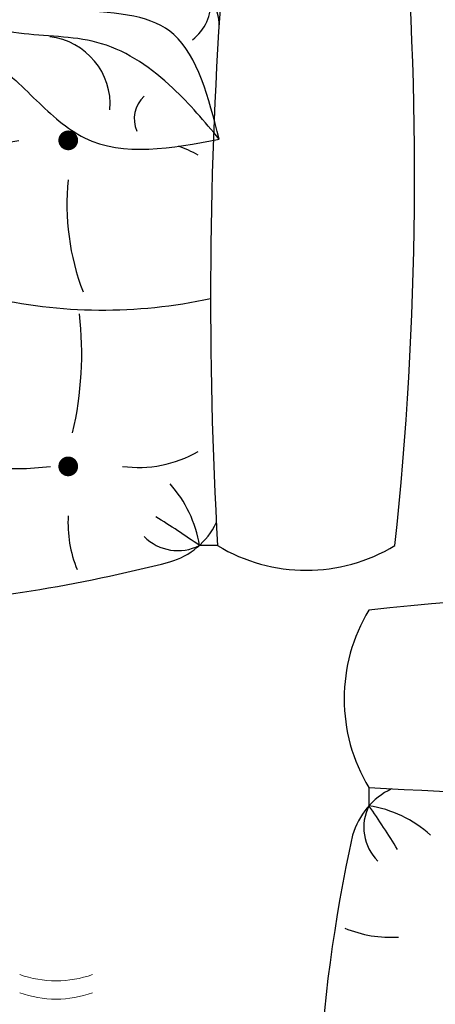
# Model space of a CAD drawing. Units: inches. Extents: x 844 to 2234, y 346 to 1084.
# Tile 88 of 93: x 2010.87 to 2017.59, y 712.93 to 728.83. Entities that reach past the tile are written whole.
import ezdxf

# ---------------------------------------------------------------- set-up
doc = ezdxf.new("R2010")
doc.units = ezdxf.units.IN
doc.header["$MEASUREMENT"] = 0
for name, color, linetype, lineweight in [('A-ANNO-DIMS', 2, 'Continuous', 18), ('furniture', 8, 'Continuous', 18), ('RA-AP-01$0$INT', 35, 'Continuous', 5)]:
    doc.layers.add(name, color=color, linetype=linetype, lineweight=lineweight)
doc.layers.add('RA-AP-01$0$FURN', color=3, linetype='Continuous')
doc.layers.add('RA-AP-01$0$WOOD', color=64, linetype='Continuous')
doc.styles.get("Standard").update_dxf_attribs({"font": 'arial.ttf'})
doc.dimstyles.get("Standard").update_dxf_attribs({"dimtxt": 6, "dimasz": 3, "dimexe": 0.18, "dimexo": 0.0625, "dimgap": 0.09, "dimtad": 0, "dimtih": 1, "dimtoh": 1, "dimdec": 1, "dimzin": 0, "dimdsep": 46, "dimlunit": 3, "dimtxsty": 'Standard', "dimblk": 'ARCHTICK', "dimcen": 0.09, "dimadec": 0, "dimazin": 0, "dimtfac": 1, "dimtdec": 1, "dimtofl": 0, "dimtmove": 0, "dimatfit": 3, "dimfxl": 1, "dimtolj": 1, "dimtzin": 0, "dimarcsym": 0})

# ---------------------------------------------------------------- blocks, each defined once
blk = doc.blocks.new('A$C7EE91E48')
at = {"layer": 'RA-AP-01$0$FURN'}
blk.add_line((9.775453681024517, -8.916612252413607), (9.757112325609974, -8.91661225241228), dxfattribs=at)
for centre, radius, start, end in [((9.387879261544771, -10.44238280163197), 1.579145581857318, 77.59199468308728, 96.58839125635443), ((9.745074433540111, -8.938971204538984), 0.1212957045587361, 157.3375839744822, 183.7314750942433), ((9.706394910853488, -8.972574909806593), 0.0753785023123622, 25.87456190605585, 73.98335472300344), ((9.865453681024029, -9.0661122524033), 0.1744999999876311, 58.95177800404677, 121.0482219959531), ((9.735181781955493, -8.959417410432842), 0.0479292786975047, 62.80708685435548, 135.4025460716553), ((9.125600268712216, -8.003664990327692), 1.11020813118073, 301.9328608597714, 304.6664773187981), ((9.636732167011939, -8.897645467382876), 0.1218651776285568, 318.0375529564433, 351.0462320954125), ((14.24233490628227, -9.167687782925107), 4.473931917517753, 176.7828902523826, 184.1477233631118), ((6.42249118116022, -9.291612252417751), 3.552808610866049, 355.0473312316413, 6.058872375658039)]:
    blk.add_arc(centre, radius, start, end, dxfattribs=at)
blk = doc.blocks.new('A$C18D01794')
at = {"layer": 'RA-AP-01$0$INT'}
for centre in [(4.309006456945037, -8.156264458284674), (4.309006456945037, -8.179364458283423)]:
    blk.add_arc(centre, 0.136414042854523, 70.20384312815696, 109.7961568705686, dxfattribs=at)
blk = doc.blocks.new('A$C7F4351E2')
at = {"layer": 'RA-AP-01$0$FURN'}
for p, q in [((8.352559572600457, -8.263941955512525), (8.35255957259913, -8.282283310927069)), ((8.352559572600457, -8.927748273106442), (8.35255957259913, -8.909406917691898))]:
    blk.add_line(p, q, dxfattribs=at)
at = {"layer": 'RA-AP-01$0$FURN', "const_width": 0.01}
for points in [[(8.437812509519787, -8.415359762755768, 1), (8.427812509519786, -8.415359762755742, 1)], [(8.758197489244363, -8.415359762756214, -1), (8.768197489244365, -8.415359762756214, -1)], [(8.437812509519787, -8.776330465863198, -1), (8.427812509519786, -8.776330465863225, -1)], [(8.758197489244363, -8.776330465862753, 1), (8.768197489244365, -8.776330465862753, 1)]]:
    blk.add_lwpolyline(points, format="xyb", close=True, dxfattribs=at)
at = {"layer": 'RA-AP-01$0$FURN'}
for centre, radius, start, end in [((8.727559572604601, -11.61690445537682), 3.552808610866049, 85.0473312316413, 96.05887237565803), ((9.025650106946005, -8.176987401637472), 0.1, 15.499494600857, 85.04733123164159), ((8.50205957259015, -8.17394195551301), 0.1744999999876311, 148.9517780040467, 211.048221995953), ((8.77247054904813, -7.958543863781743), 0.3382138395168437, 297.2303327094027, 328.2563708342649), ((9.2484631175852, -8.302692737637487), 0.3241573581843151, 149.2985674842688, 172.3026350986055), ((7.88981694267423, -8.595845114309485), 1.310286319972027, 340.1192502251003, 19.8807497748998), ((9.084915705374858, -8.196040134964925), 0.1698955038956699, 168.877843135945, 201.8512383801196), ((7.929864357850293, -8.595845114309483), 1.224941341589781, 341.1257460634955, 18.87425393650447), ((8.947672844970796, -8.191835192646359), 0.0704710051510922, 253.1338634205325, 306.4126496157095), ((8.603635103111959, -3.79706073025477), 4.473931917517753, 266.7828902523826, 274.1477233631118), ((10.52713941284929, -8.595845114309466), 1.634931324962266, 168.1200364254424, 191.8799635745573), ((8.408522229993444, -8.33300072568355), 0.0753785023123622, 115.8745619060558, 163.9833547230034), ((9.101231010340802, -8.38034106221356), 0.5100538472773755, 167.6182489359307, 193.3122231353938), ((8.903279781571525, -8.31837865610295), 0.0478550828899777, 86.575295631534, 142.6833829238214), ((8.878389979098333, -8.312202545234353), 0.05, 30.14777190425723, 89.99999999905349), ((8.838100984994732, -8.276822957859652), 0.0683206773889159, 326.6729861493449, 5.218395042636973), ((8.810121490949696, -8.31110757721543), 0.1042084262671507, 340.4828318717155, 22.86929393278168), ((8.395364730619693, -8.304213854581548), 0.0479292786975047, 152.8070868543555, 225.4025460716553), ((8.333592787569726, -8.402663469525104), 0.1218651776285568, 48.0375529564433, 81.04623209541253), ((7.439612310514541, -8.913795367824825), 1.11020813118073, 31.93286085977143, 34.66647731879807), ((8.553131949433, -8.344109762755968), 0.1214118203512435, 150.1419074485596, 187.691663289156), ((8.642878049331348, -8.344109762756093), 0.1214118203512435, 352.3083367106845, 29.85809255128089), ((9.82633505008426, -8.696671375220811), 1.539060359583382, 165.5338783218257, 176.2437734318419), ((8.697701155637269, -8.172468128267624), 0.2442261434243043, 248.9017070735605, 275.9923925191661), ((8.374918524725835, -8.294321202996931), 0.1212957045587361, 247.3375839744822, 273.7314750942433), ((8.546954810732721, -8.753394424755975), 0.3517162425384579, 83.41248966761125, 103.1674570565571), ((8.73287643248165, -8.469775898206471), 0.3023568492824586, 173.0944825511667, 197.588060785551), ((8.889871101981017, -8.492307869305423), 0.1295083186917369, 167.9901339202812, 211.3796151021958), ((8.444145567704187, -7.829943385268752), 0.765467899454341, 258.6273206109321, 281.4174148186357), ((8.781211457338294, -7.772561243483908), 0.8232838708255751, 260.2449188973366, 277.7495311655964), ((9.82633505008426, -8.495018853398156), 1.539060359583382, 183.7562265681581, 194.4661216781742), ((8.444145567704187, -9.361312955433425), 0.765467899454341, 78.58258518136427, 101.3726793890678), ((8.781211457338294, -9.418695097218269), 0.8232838708255751, 82.25060502413102, 99.75508110266344), ((8.73287643248165, -8.721914330412496), 0.3023568492824586, 162.411939214449, 186.9055174488332), ((8.889871101981017, -8.699382359313544), 0.1295083186917369, 148.6203848978042, 192.0098660797188), ((9.101231010340802, -8.811349166405407), 0.5100538472773755, 166.6877768646062, 192.3817510640693), ((8.799643412436344, -8.749969313933361), 0.0689028341546707, 265.5384273543114, 353.5804828909086), ((8.374918524725835, -8.897369025622035), 0.1212957045587361, 86.26852490575668, 112.6624160255178), ((8.697701155637269, -9.019222100351342), 0.2442261434243043, 84.00760748083387, 111.0982929264395), ((8.546954810732721, -8.438295803862992), 0.3517162425384579, 256.8325429434429, 276.5875103323888), ((8.553131949433, -8.847580465862999), 0.1214118203512435, 172.308336710844, 209.8580925514404), ((8.785133372574222, -8.874256642962408), 0.0310151388417235, 42.62105484496073, 114.2239681486109), ((8.810121490949696, -8.880582651403534), 0.1042084262671507, 337.1307060672183, 19.51716812828453), ((8.395364730619693, -8.88747637403742), 0.0479292786975047, 134.5974539283447, 207.1929131456445), ((7.439612310514541, -8.277894860794142), 1.11020813118073, 325.333522681202, 328.0671391402286), ((8.408522229993444, -8.858689502935416), 0.0753785023123622, 196.0166452769965, 244.1254380939442), ((8.333592787569726, -8.789026759093863), 0.1218651776285568, 278.9537679045875, 311.9624470435567), ((8.838100984994732, -8.914867270759315), 0.0683206773889159, 354.781604957363, 33.32701385065517), ((8.642878049331348, -8.847580465862874), 0.1214118203512435, 330.1419074487191, 340.3913536181062), ((8.878389979098333, -8.879487683384612), 0.05, 270.0000000009465, 337.4173275753961), ((8.903279781571525, -8.873311572516016), 0.0478550828899777, 217.3166170761785, 273.424704368466), ((8.50205957259015, -9.017748273105955), 0.1744999999876311, 148.9517780040469, 211.0482219959533), ((8.603635103111959, -13.39462949836419), 4.473931917517753, 85.85227663688822, 93.21710974761734), ((8.947672844970796, -8.999855035972608), 0.0704710051510922, 53.58735038429053, 106.8661365794674), ((9.084915705374858, -8.995650093654042), 0.1698955038956699, 158.1487616198804, 191.122156864055), ((8.77247054904813, -9.233146364837223), 0.3382138395168437, 31.74362916573515, 62.76966729059727), ((9.2484631175852, -8.88899749098148), 0.3241573581843151, 187.6973649013944, 210.7014325157311), ((9.025650106946005, -9.014702826981493), 0.1, 274.9526687683584, 344.500505399143), ((8.727559572604601, -5.574785773242145), 3.552808610866049, 263.941127624342, 274.9526687683587)]:
    blk.add_arc(centre, radius, start, end, dxfattribs=at)
for points, knots in [([(8.764421239581775, -8.929562504990262), (8.755250524728652, -8.881106864374377), (8.74196437992213, -8.810906376383404), (8.80604948961138, -8.740469753734786), (8.847474678848357, -8.701097198289744), (8.897142214037096, -8.58322730303861), (8.897091569728207, -8.784804210134517), (8.88612504526093, -8.897825917224484), (8.806539053396843, -8.9185794820093), (8.764421239581775, -8.92956250499026)], [0, 0, 0, 0, 0.1367586589314792, 0.1981301758052368, 0.2677729570689282, 0.3281194902553322, 0.4737578340741565, 0.5765194025309516, 0.6920332287422236, 0.6920332287422236, 0.6920332287422236, 0.6920332287422236]), ([(8.764421239581775, -8.92956250499026), (8.782204778269502, -8.914603263160053), (8.821592007255505, -8.881471326160916), (8.86917941606436, -8.814322636989944), (8.867818990542759, -8.729338202119969), (8.881231406199264, -8.676770566934765), (8.888101821971249, -8.649843164808122)], [0, 0, 0, 0, 0.070018540671015, 0.1550780383534498, 0.2344491945777043, 0.3178048737568289, 0.3178048737568289, 0.3178048737568289, 0.3178048737568289])]:
    blk.add_open_spline(points, degree=3, knots=knots, dxfattribs=at)
blk = doc.blocks.new('A$C5D2F253E')
at = {"layer": 'RA-AP-01$0$FURN', "xscale": -0.7999999999883585, "yscale": 0.7999999999883585, "zscale": 0.8, "rotation": 90}
blk.add_blockref('A$C18D01794', (-5.687757199772477, 4.75791982714071), dxfattribs=at)
at = {"layer": 'RA-AP-01$0$WOOD', "xscale": -1, "rotation": 180}
for name, p in [('A$C7EE91E48', (-8.833013809079146, -7.288751725733902)), ('A$C7F4351E2', (-7.164808785335935, -7.45332973198748))]:
    blk.add_blockref(name, p, dxfattribs=at)
blk = doc.blocks.new('_ArchTick')
at = {"color": 0, "linetype": 'ByBlock', "const_width": 0.15}
blk.add_lwpolyline([(-0.5, -0.5), (0.5, 0.5)], dxfattribs=at)
blk = doc.blocks.new('*D121')
at = {"layer": 'A-ANNO-DIMS', "color": 0, "lineweight": -2, "transparency": 16777216}
for p, q in [((2030.271987351997, 734.262611118704), (2040.245275089302, 734.262611118704)), ((2040.065275089302, 734.262611118704), (2040.065275089302, 704.6043509484256)), ((2040.065275089302, 668.557359536674), (2040.065275089302, 698.2156197069523)), ((2030.271987351997, 668.557359536674), (2040.245275089302, 668.557359536674))]:
    blk.add_line(p, q, dxfattribs=at)
at = {"layer": 'Defpoints', "color": 0, "transparency": 16777216}
for p in [(2030.209487351997, 734.262611118704), (2040.065275089302, 734.262611118704), (2030.209487351997, 668.557359536674)]:
    blk.add_point(p, dxfattribs=at)
at = {"layer": 'A-ANNO-DIMS', "color": 0, "lineweight": -2, "transparency": 16777216, "xscale": 3, "yscale": 3, "zscale": 3}
for p, rotation in [((2040.065275089302, 734.262611118704), 90), ((2040.065275089302, 668.557359536674), 270)]:
    blk.add_blockref('_ArchTick', p, dxfattribs=dict(at, rotation=rotation))
at = {"layer": 'A-ANNO-DIMS', "color": 0, "transparency": 16777216, "insert": (2040.065275089302, 701.4099853276883), "char_height": 6, "attachment_point": 5}
blk.add_mtext('\\A1;LOUNGE SET 5\'-5 1/2" TYP.', dxfattribs=at)

msp = doc.modelspace()

# ---------------------------------------------------------------- block references
at = {"layer": 'furniture', "xscale": -15.94108302203742, "yscale": 15.94108302203742, "zscale": 15.94108302203742, "rotation": 270}
msp.add_blockref('A$C5D2F253E', (1990.567271852805, 701.4028671565849), dxfattribs=at)

# ---------------------------------------------------------------- dimensions: what is measured, and where the dimension line sits
at = {"layer": 'A-ANNO-DIMS'}
dim = msp.add_linear_dim(base=(2040.065275089302, 734.262611118704), p1=(2030.209487351996, 668.5573595366737), p2=(2030.209487351996, 734.2626111187037), angle=90, text='LOUNGE SET <> TYP.', dimstyle='Standard', override={"dimdec": 1, "dimlfac": 1, "dimrnd": 0, "dimzin": 1, "dimdsep": 46, "dimlunit": 4, "dimfrac": 2}, dxfattribs=at)
dim.commit()
dim.dimension.update_dxf_attribs({"geometry": '*D121', "text_midpoint": (2040.065275089302, 701.4099853276883)})

doc.saveas('drawing.dxf')
